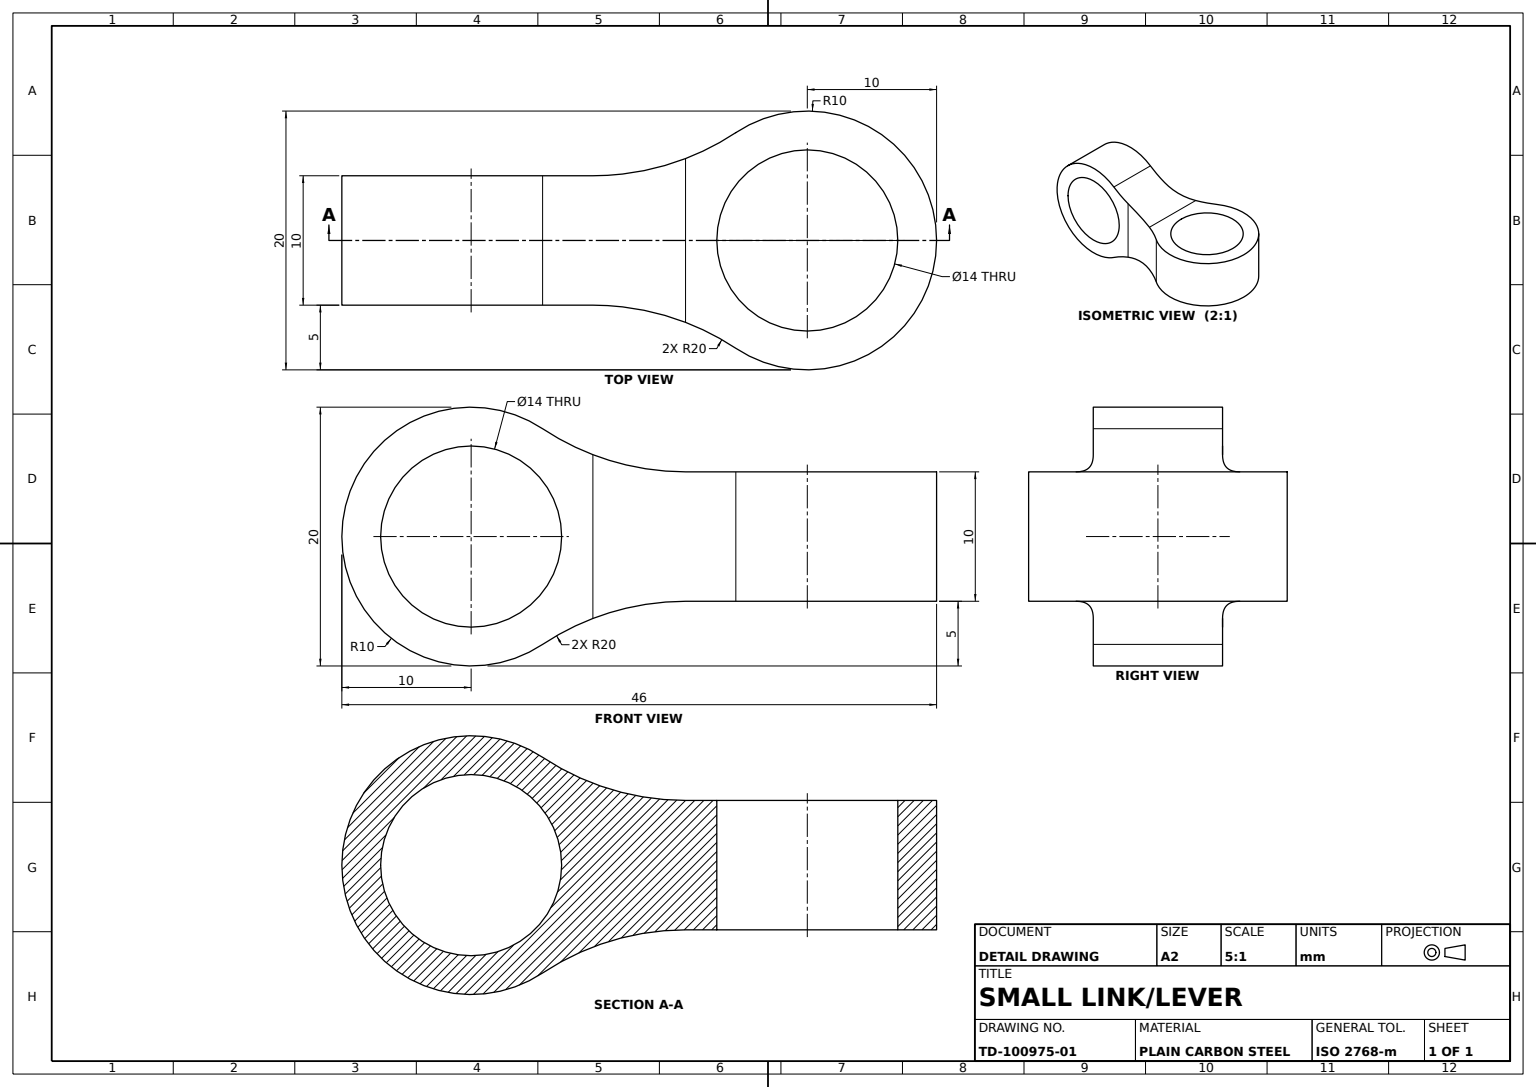
from build123d import *

# Parameters (mm, degrees)
LINK_BLOCK_SKETCH_W               = 46
LINK_BLOCK_SKETCH_H               = 20
LINK_BLOCK_DEPTH                  = 10
FIRST_LUG_PROFILE_SKETCH_R        = 7
FIRST_LUG_PROFILE_BORE_CUT_DEPTH  = 35
SECOND_LUG_PROFILE_SKETCH_W       = 55.121968116
SECOND_LUG_PROFILE_SKETCH_H       = 28.549832612
SECOND_LUG_PROFILE_SKETCH_R       = 7
SECOND_LUG_PROFILE_BORE_CUT_DEPTH = 35


with BuildPart() as part:
    # Link Block Sketch → Link Block (new, symmetric)
    with BuildSketch(Plane.XY):
        Rectangle(LINK_BLOCK_SKETCH_W, LINK_BLOCK_SKETCH_H)
    extrude(amount=LINK_BLOCK_DEPTH, both=True)

    # First Lug Profile Sketch → First Lug Profile & Bore Cut (cut, symmetric)
    with BuildSketch(Plane.XY.offset(10)):
        with BuildLine():
            ThreePointArc((-7.472292016, 8.333333333), (-2.19037874, 5.851457845), (3.583123952, 5))
            Line((3.583123952, 5), (23, 5))
            Line((23, 5), (23, 10))
            Line((23, 10), (-13, 10))
            ThreePointArc((-13, 10), (-10.113248654, 9.574271078), (-7.472292016, 8.333333333))
        make_face()
        with BuildLine():
            ThreePointArc((-23, -4.3e-08), (-20.071067827, 7.071067797), (-13, 10))
            Line((-13, 10), (-23, 10))
            Line((-23, 10), (-23, -4.3e-08))
        make_face()
        with BuildLine():
            ThreePointArc((-13, -10), (-20.071067797, -7.071067827), (-23, -4.3e-08))
            Line((-23, -4.3e-08), (-23, -10))
            Line((-23, -10), (-13, -10))
        make_face()
        with BuildLine():
            Line((23, -10), (23, -5))
            Line((23, -5), (3.583123952, -5))
            ThreePointArc((3.583123952, -5), (-2.19037874, -5.851457845), (-7.472292016, -8.333333333))
            ThreePointArc((-7.472292016, -8.333333333), (-10.113248654, -9.574271078), (-13, -10))
            Line((-13, -10), (23, -10))
        make_face()
        with Locations((-13, 0)):
            Circle(FIRST_LUG_PROFILE_SKETCH_R)
    extrude(amount=FIRST_LUG_PROFILE_BORE_CUT_DEPTH, both=True, mode=Mode.SUBTRACT)

    # Second Lug Profile Sketch → Second Lug Profile & Bore Cut (cut, symmetric)
    # profile 1 of 6: a face of its own
    with BuildSketch(Plane.XZ.offset(5)):
        with Locations((1.394530012, 1.140979101)):
            Rectangle(SECOND_LUG_PROFILE_SKETCH_W, SECOND_LUG_PROFILE_SKETCH_H)
        with BuildLine():
            Line((-23, -5), (-23, 5))
            Line((-23, 5), (-3.583123952, 5))
            ThreePointArc((-3.583123952, 5), (0.06100146, 5.334793416), (3.583123952, 6.327965002))
            Line((3.583123952, 6.327965002), (3.583123952, 10))
            Line((3.583123952, 10), (13, 10))
            Line((13, 10), (23, 10))
            Line((23, 10), (23, -6e-08))
            Line((23, -6e-08), (23, -10))
            Line((23, -10), (12.999999984, -10))
            Line((12.999999984, -10), (3.583123952, -10))
            Line((3.583123952, -10), (3.583123952, -6.327965002))
            ThreePointArc((3.583123952, -6.327965002), (0.06100146, -5.334793416), (-3.583123952, -5))
            Line((-3.583123952, -5), (-23, -5))
        make_face(mode=Mode.SUBTRACT)
    # profile 2 of 6: a face of its own
    with BuildSketch(Plane.XZ.offset(5)):
        with Locations((13, 0)):
            Circle(SECOND_LUG_PROFILE_SKETCH_R)
    # profile 3 of 6: a face of its own
    with BuildSketch(Plane.XZ.offset(5)):
        with BuildLine():
            Line((23, -10), (23, -6e-08))
            ThreePointArc((23, -6e-08), (20.071067785, -7.071067839), (12.999999984, -10))
            Line((12.999999984, -10), (23, -10))
        make_face()
    # profile 4 of 6: a face of its own
    with BuildSketch(Plane.XZ.offset(5)):
        with BuildLine():
            ThreePointArc((7.472292016, -8.333333333), (5.582716659, -7.223966531), (3.583123952, -6.327965002))
            Line((3.583123952, -6.327965002), (3.583123952, -10))
            Line((3.583123952, -10), (12.999999984, -10))
            ThreePointArc((12.999999984, -10), (10.113248646, -9.574271075), (7.472292016, -8.333333333))
        make_face()
    # profile 5 of 6: a face of its own
    with BuildSketch(Plane.XZ.offset(5)):
        with BuildLine():
            Line((3.583123952, 10), (3.583123952, 6.327965002))
            ThreePointArc((3.583123952, 6.327965002), (5.582716659, 7.223966531), (7.472292016, 8.333333333))
            ThreePointArc((7.472292016, 8.333333333), (10.113248654, 9.574271078), (13, 10))
            Line((13, 10), (3.583123952, 10))
        make_face()
    # profile 6 of 6: a face of its own
    with BuildSketch(Plane.XZ.offset(5)):
        with BuildLine():
            Line((23, 10), (13, 10))
            ThreePointArc((13, 10), (20.071067833, 7.071067791), (23, -6e-08))
            Line((23, -6e-08), (23, 10))
        make_face()
    extrude(amount=SECOND_LUG_PROFILE_BORE_CUT_DEPTH, both=True, mode=Mode.SUBTRACT)


solid = part.part
